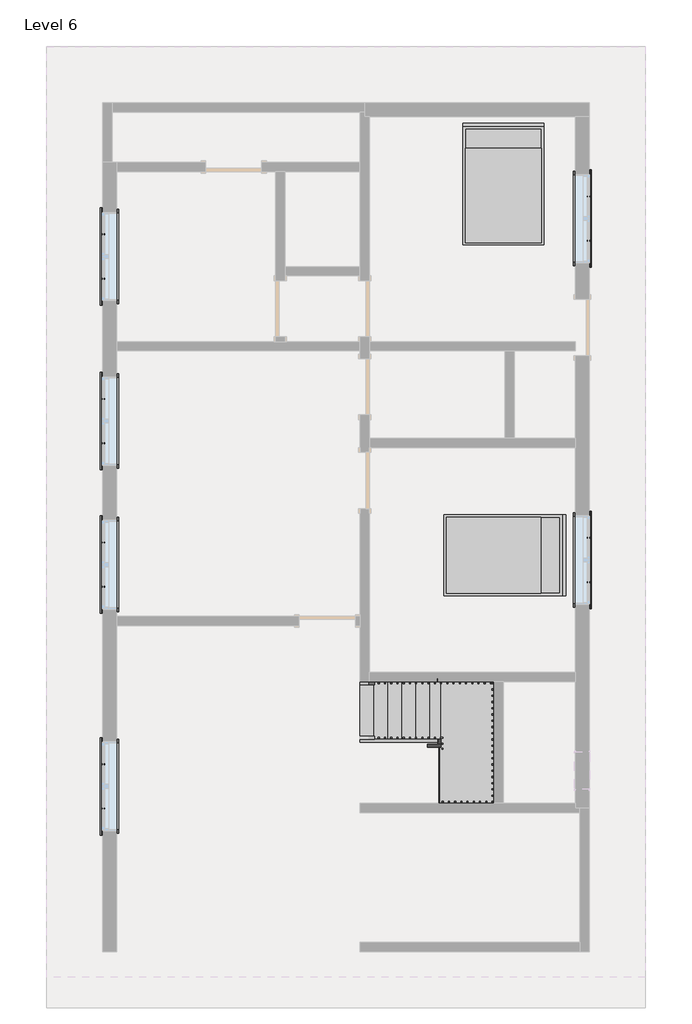
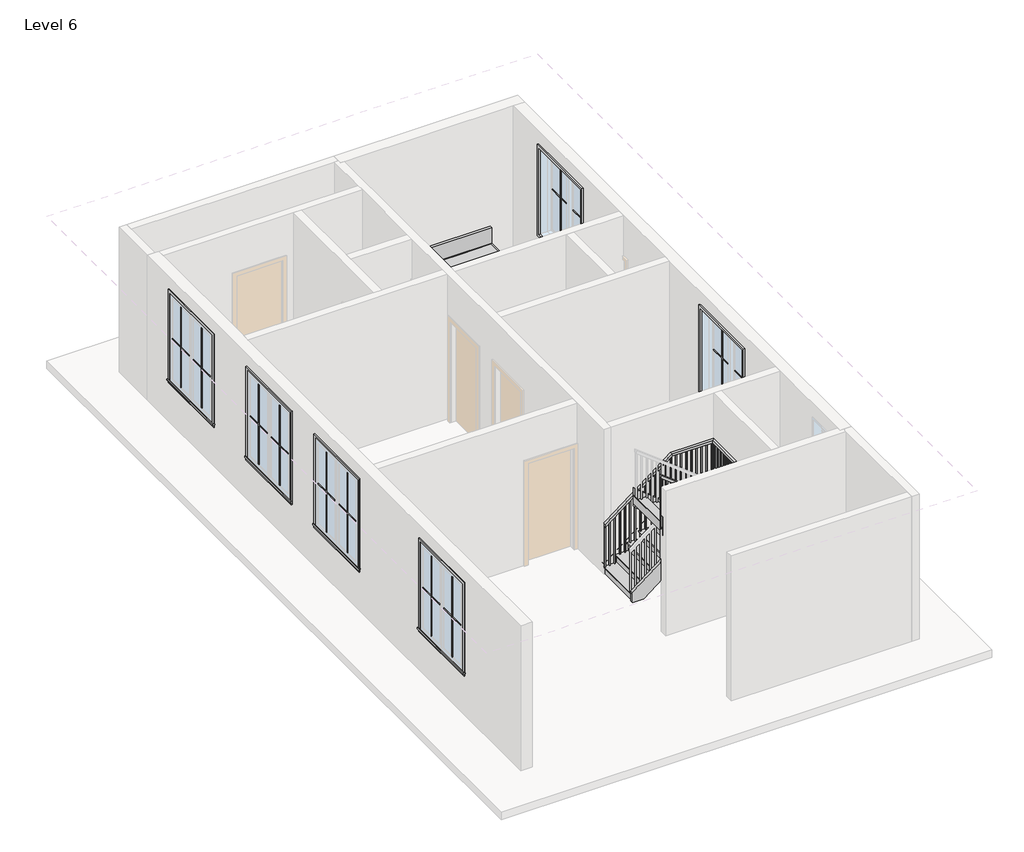
# One storey, part 2 of 2: 24 proxies, 6 members, 2 furniture elements, 1 railing, 1 stair flight.
"""IFC4 building model written with IfcOpenShell, lengths in millimetres."""

from ifc_helpers import new_model, si_unit, frame, origin, place, context, project, spatial, polyline, outline, extrude, faceted_brep, transform, mapped, element, save
from components import muntin_pattern_2x2_muntin_pattern_2x2_bff912c5, muntin_pattern_2x2_muntin_pattern_2x2_c2194282, trim_window_exterior_flat_with_sill_e04b3088, trim_window_interior_flat_picture_frame_2a7685fe, bed_17739_bed_17739_15c61121, stair_flight_b066332a

model = new_model("IFC4")

# Units and contexts
model_context = context("Model", 3, world=origin())
ifc_project = project(units=[si_unit("LENGTHUNIT", "METRE", prefix="MILLI")], contexts=[model_context])

# Site, building, storey
site = spatial("IfcSite", under=ifc_project)
building = spatial("IfcBuilding", under=site)
storey = spatial("IfcBuildingStorey", under=building, Name="Level 6", Elevation=12801.6)

# Proxies
placement = place(None, origin())
muntin_pattern_2x2_muntin_pattern_2x2_shape = muntin_pattern_2x2_muntin_pattern_2x2_bff912c5(model_context)
element("IfcBuildingElementProxy", 1, Name="Muntin Pattern_2x2 : Muntin Pattern_2x2", ObjectType="Muntin Pattern_2x2 : Muntin Pattern_2x2", at=placement, inside=storey, context=model_context, shape_type="MappedRepresentation", body=[
    mapped(muntin_pattern_2x2_muntin_pattern_2x2_shape, transform((-5204.1165352, 3633.8812696, 13785.85), x_axis=(0.0, 1.0, 0.0), y_axis=(-1.0, 0.0, 0.0), z_axis=(0.0, 0.0, 1.0))),
])
element("IfcBuildingElementProxy", 2, Name="Muntin Pattern_2x2 : Muntin Pattern_2x2", ObjectType="Muntin Pattern_2x2 : Muntin Pattern_2x2", at=placement, inside=storey, context=model_context, shape_type="MappedRepresentation", body=[
    mapped(muntin_pattern_2x2_muntin_pattern_2x2_shape, transform((2701.6334648, 4971.3355313, 13785.85), x_axis=(0.0, -1.0, 0.0), y_axis=(1.0, 0.0, 0.0), z_axis=(0.0, 0.0, 1.0))),
])
element("IfcBuildingElementProxy", 3, Name="Muntin Pattern_2x2 : Muntin Pattern_2x2", ObjectType="Muntin Pattern_2x2 : Muntin Pattern_2x2", at=placement, inside=storey, context=model_context, shape_type="MappedRepresentation", body=[
    mapped(muntin_pattern_2x2_muntin_pattern_2x2_shape, transform((2701.6334648, -584.9144687, 13785.85), x_axis=(0.0, -1.0, 0.0), y_axis=(1.0, 0.0, 0.0), z_axis=(0.0, 0.0, 1.0))),
])
element("IfcBuildingElementProxy", 4, Name="Muntin Pattern_2x2 : Muntin Pattern_2x2", ObjectType="Muntin Pattern_2x2 : Muntin Pattern_2x2", at=placement, inside=storey, context=model_context, shape_type="MappedRepresentation", body=[
    mapped(muntin_pattern_2x2_muntin_pattern_2x2_shape, transform((-5204.1165352, 954.9605313, 13785.85), x_axis=(0.0, 1.0, 0.0), y_axis=(-1.0, 0.0, 0.0), z_axis=(0.0, 0.0, 1.0))),
])
element("IfcBuildingElementProxy", 5, Name="Muntin Pattern_2x2 : Muntin Pattern_2x2", ObjectType="Muntin Pattern_2x2 : Muntin Pattern_2x2", at=placement, inside=storey, context=model_context, shape_type="MappedRepresentation", body=[
    mapped(muntin_pattern_2x2_muntin_pattern_2x2_shape, transform((-5204.1165352, -1381.8394687, 13785.85), x_axis=(0.0, 1.0, 0.0), y_axis=(-1.0, 0.0, 0.0), z_axis=(0.0, 0.0, 1.0))),
])
element("IfcBuildingElementProxy", 6, Name="Muntin Pattern_2x2 : Muntin Pattern_2x2", ObjectType="Muntin Pattern_2x2 : Muntin Pattern_2x2", at=placement, inside=storey, context=model_context, shape_type="MappedRepresentation", body=[
    mapped(muntin_pattern_2x2_muntin_pattern_2x2_shape, transform((-5204.1165352, -4988.6394687, 13785.85), x_axis=(0.0, 1.0, 0.0), y_axis=(-1.0, 0.0, 0.0), z_axis=(0.0, 0.0, 1.0))),
])
muntin_pattern_2x2_muntin_pattern_2x2_2_shape = muntin_pattern_2x2_muntin_pattern_2x2_c2194282(model_context)
element("IfcBuildingElementProxy", 7, Name="Muntin Pattern_2x2 : Muntin Pattern_2x2", ObjectType="Muntin Pattern_2x2 : Muntin Pattern_2x2", at=placement, inside=storey, context=model_context, shape_type="MappedRepresentation", body=[
    mapped(muntin_pattern_2x2_muntin_pattern_2x2_2_shape, transform((-5204.1165352, 4354.6062696, 13785.85), x_axis=(0.0, -1.0, 0.0), y_axis=(1.0, 0.0, 0.0), z_axis=(0.0, 0.0, 1.0))),
])
element("IfcBuildingElementProxy", 8, Name="Muntin Pattern_2x2 : Muntin Pattern_2x2", ObjectType="Muntin Pattern_2x2 : Muntin Pattern_2x2", at=placement, inside=storey, context=model_context, shape_type="MappedRepresentation", body=[
    mapped(muntin_pattern_2x2_muntin_pattern_2x2_2_shape, transform((2701.6334648, 4250.6105313, 13785.85), x_axis=(0.0, 1.0, 0.0), y_axis=(-1.0, 0.0, 0.0), z_axis=(0.0, 0.0, 1.0))),
])
element("IfcBuildingElementProxy", 9, Name="Muntin Pattern_2x2 : Muntin Pattern_2x2", ObjectType="Muntin Pattern_2x2 : Muntin Pattern_2x2", at=placement, inside=storey, context=model_context, shape_type="MappedRepresentation", body=[
    mapped(muntin_pattern_2x2_muntin_pattern_2x2_2_shape, transform((2701.6334648, -1305.6394687, 13785.85), x_axis=(0.0, 1.0, 0.0), y_axis=(-1.0, 0.0, 0.0), z_axis=(0.0, 0.0, 1.0))),
])
element("IfcBuildingElementProxy", 10, Name="Muntin Pattern_2x2 : Muntin Pattern_2x2", ObjectType="Muntin Pattern_2x2 : Muntin Pattern_2x2", at=placement, inside=storey, context=model_context, shape_type="MappedRepresentation", body=[
    mapped(muntin_pattern_2x2_muntin_pattern_2x2_2_shape, transform((-5204.1165352, 1675.6855313, 13785.85), x_axis=(0.0, -1.0, 0.0), y_axis=(1.0, 0.0, 0.0), z_axis=(0.0, 0.0, 1.0))),
])
element("IfcBuildingElementProxy", 11, Name="Muntin Pattern_2x2 : Muntin Pattern_2x2", ObjectType="Muntin Pattern_2x2 : Muntin Pattern_2x2", at=placement, inside=storey, context=model_context, shape_type="MappedRepresentation", body=[
    mapped(muntin_pattern_2x2_muntin_pattern_2x2_2_shape, transform((-5204.1165352, -661.1144687, 13785.85), x_axis=(0.0, -1.0, 0.0), y_axis=(1.0, 0.0, 0.0), z_axis=(0.0, 0.0, 1.0))),
])
element("IfcBuildingElementProxy", 12, Name="Muntin Pattern_2x2 : Muntin Pattern_2x2", ObjectType="Muntin Pattern_2x2 : Muntin Pattern_2x2", at=placement, inside=storey, context=model_context, shape_type="MappedRepresentation", body=[
    mapped(muntin_pattern_2x2_muntin_pattern_2x2_2_shape, transform((-5204.1165352, -4267.9144687, 13785.85), x_axis=(0.0, -1.0, 0.0), y_axis=(1.0, 0.0, 0.0), z_axis=(0.0, 0.0, 1.0))),
])
trim_window_exterior_flat_with_sill_shape = trim_window_exterior_flat_with_sill_e04b3088(model_context)
element("IfcBuildingElementProxy", 13, Name="Trim-Window-Exterior-Flat : with Sill", ObjectType="Trim-Window-Exterior-Flat : with Sill", at=placement, inside=storey, context=model_context, shape_type="MappedRepresentation", body=[
    mapped(trim_window_exterior_flat_with_sill_shape, transform((-5213.6415352, 3994.2437696, 15544.8), x_axis=(0.0, -1.0, 0.0), y_axis=(0.0, 0.0, 1.0), z_axis=(-1.0, 0.0, 0.0))),
])
element("IfcBuildingElementProxy", 14, Name="Trim-Window-Exterior-Flat : with Sill", ObjectType="Trim-Window-Exterior-Flat : with Sill", at=placement, inside=storey, context=model_context, shape_type="MappedRepresentation", body=[
    mapped(trim_window_exterior_flat_with_sill_shape, transform((2711.1584648, 4610.9730313, 15544.8), x_axis=(0.0, 1.0, 0.0), y_axis=(0.0, 0.0, 1.0), z_axis=(1.0, 0.0, 0.0))),
])
element("IfcBuildingElementProxy", 15, Name="Trim-Window-Exterior-Flat : with Sill", ObjectType="Trim-Window-Exterior-Flat : with Sill", at=placement, inside=storey, context=model_context, shape_type="MappedRepresentation", body=[
    mapped(trim_window_exterior_flat_with_sill_shape, transform((2711.1584648, -945.2769687, 15544.8), x_axis=(0.0, 1.0, 0.0), y_axis=(0.0, 0.0, 1.0), z_axis=(1.0, 0.0, 0.0))),
])
element("IfcBuildingElementProxy", 16, Name="Trim-Window-Exterior-Flat : with Sill", ObjectType="Trim-Window-Exterior-Flat : with Sill", at=placement, inside=storey, context=model_context, shape_type="MappedRepresentation", body=[
    mapped(trim_window_exterior_flat_with_sill_shape, transform((-5213.6415352, 1315.3230313, 15544.8), x_axis=(0.0, -1.0, 0.0), y_axis=(0.0, 0.0, 1.0), z_axis=(-1.0, 0.0, 0.0))),
])
element("IfcBuildingElementProxy", 17, Name="Trim-Window-Exterior-Flat : with Sill", ObjectType="Trim-Window-Exterior-Flat : with Sill", at=placement, inside=storey, context=model_context, shape_type="MappedRepresentation", body=[
    mapped(trim_window_exterior_flat_with_sill_shape, transform((-5213.6415352, -1021.4769687, 15544.8), x_axis=(0.0, -1.0, 0.0), y_axis=(0.0, 0.0, 1.0), z_axis=(-1.0, 0.0, 0.0))),
])
element("IfcBuildingElementProxy", 18, Name="Trim-Window-Exterior-Flat : with Sill", ObjectType="Trim-Window-Exterior-Flat : with Sill", at=placement, inside=storey, context=model_context, shape_type="MappedRepresentation", body=[
    mapped(trim_window_exterior_flat_with_sill_shape, transform((-5213.6415352, -4628.2769687, 15544.8), x_axis=(0.0, -1.0, 0.0), y_axis=(0.0, 0.0, 1.0), z_axis=(-1.0, 0.0, 0.0))),
])
trim_window_interior_flat_picture_frame_shape = trim_window_interior_flat_picture_frame_2a7685fe(model_context)
element("IfcBuildingElementProxy", 19, Name="Trim-Window-Interior-Flat : Picture Frame", ObjectType="Trim-Window-Interior-Flat : Picture Frame", at=placement, inside=storey, context=model_context, shape_type="MappedRepresentation", body=[
    mapped(trim_window_interior_flat_picture_frame_shape, transform((-4985.0415352, 3994.2437696, 15544.8), x_axis=(0.0, 1.0, 0.0), y_axis=(0.0, 0.0, 1.0), z_axis=(1.0, 0.0, 0.0))),
])
element("IfcBuildingElementProxy", 20, Name="Trim-Window-Interior-Flat : Picture Frame", ObjectType="Trim-Window-Interior-Flat : Picture Frame", at=placement, inside=storey, context=model_context, shape_type="MappedRepresentation", body=[
    mapped(trim_window_interior_flat_picture_frame_shape, transform((2482.5584648, 4610.9730313, 15544.8), x_axis=(0.0, -1.0, 0.0), y_axis=(0.0, 0.0, 1.0), z_axis=(-1.0, 0.0, 0.0))),
])
element("IfcBuildingElementProxy", 21, Name="Trim-Window-Interior-Flat : Picture Frame", ObjectType="Trim-Window-Interior-Flat : Picture Frame", at=placement, inside=storey, context=model_context, shape_type="MappedRepresentation", body=[
    mapped(trim_window_interior_flat_picture_frame_shape, transform((2482.5584648, -945.2769687, 15544.8), x_axis=(0.0, -1.0, 0.0), y_axis=(0.0, 0.0, 1.0), z_axis=(-1.0, 0.0, 0.0))),
])
element("IfcBuildingElementProxy", 22, Name="Trim-Window-Interior-Flat : Picture Frame", ObjectType="Trim-Window-Interior-Flat : Picture Frame", at=placement, inside=storey, context=model_context, shape_type="MappedRepresentation", body=[
    mapped(trim_window_interior_flat_picture_frame_shape, transform((-4985.0415352, 1315.3230313, 15544.8), x_axis=(0.0, 1.0, 0.0), y_axis=(0.0, 0.0, 1.0), z_axis=(1.0, 0.0, 0.0))),
])
element("IfcBuildingElementProxy", 23, Name="Trim-Window-Interior-Flat : Picture Frame", ObjectType="Trim-Window-Interior-Flat : Picture Frame", at=placement, inside=storey, context=model_context, shape_type="MappedRepresentation", body=[
    mapped(trim_window_interior_flat_picture_frame_shape, transform((-4985.0415352, -1021.4769687, 15544.8), x_axis=(0.0, 1.0, 0.0), y_axis=(0.0, 0.0, 1.0), z_axis=(1.0, 0.0, 0.0))),
])
element("IfcBuildingElementProxy", 24, Name="Trim-Window-Interior-Flat : Picture Frame", ObjectType="Trim-Window-Interior-Flat : Picture Frame", at=placement, inside=storey, context=model_context, shape_type="MappedRepresentation", body=[
    mapped(trim_window_interior_flat_picture_frame_shape, transform((-4985.0415352, -4628.2769687, 15544.8), x_axis=(0.0, 1.0, 0.0), y_axis=(0.0, 0.0, 1.0), z_axis=(1.0, 0.0, 0.0))),
])

# Furniture
bed_17739_bed_17739_shape = bed_17739_bed_17739_15c61121(model_context)
element("IfcFurniture", 25, ObjectType="Bed_17739 : Bed_17739", at=placement, inside=storey, context=model_context, shape_type="MappedRepresentation", body=[
    mapped(bed_17739_bed_17739_shape, transform((1314.1584648, 5149.1645078, 12801.6), x_axis=(1.0, 0.0, 0.0), y_axis=(0.0, 1.0, 0.0), z_axis=(0.0, 0.0, 1.0))),
])
element("IfcFurniture", 26, ObjectType="Bed_17739 : Bed_17739", at=placement, inside=storey, context=model_context, shape_type="MappedRepresentation", body=[
    mapped(bed_17739_bed_17739_shape, transform((1314.1584648, -869.0769687, 12801.6), x_axis=(0.0, -1.0, 0.0), y_axis=(1.0, 0.0, 0.0), z_axis=(0.0, 0.0, 1.0))),
])

# Members
element("IfcMember", 27, ObjectType="Stringer - 2\" Width", at=placement, inside=storey, context=model_context, shape_type="SweptSolid", body=[
    extrude(outline(polyline([(13023.3399812, -1022.6415352), (12801.6, -1022.6415352), (12801.6, -811.2687863), (14063.1333333, 810.8400359), (14063.1333333, 314.3488758), (13023.3399812, -1022.6415352)])), frame((0.0, -2926.4769687, 0.0), z_axis=(0.0, 1.0, 0.0), x_axis=(0.0, 0.0, 1.0)), (0.0, 0.0, 1.0), 50.8),
])
element("IfcMember", 28, ObjectType="Stringer - 2\" Width", at=placement, inside=storey, context=model_context, shape_type="SweptSolid", body=[
    extrude(outline(polyline([(1161.7584648, -2875.6769687), (1212.5584648, -2875.6769687), (1212.5584648, -4907.6769687), (1161.7584648, -4907.6769687), (1161.7584648, -2875.6769687)])), frame((0.0, 0.0, 13758.3333333), z_axis=(0.0, 0.0, 1.0), x_axis=(1.0, 0.0, 0.0)), (0.0, 0.0, 1.0), 304.8),
])
element("IfcMember", 29, ObjectType="Stringer - 2\" Width", at=placement, inside=storey, context=model_context, shape_type="SweptSolid", body=[
    extrude(outline(polyline([(13758.3333333, 884.5469698), (15241.5765283, -1022.6415352), (14855.4494451, -1022.6415352), (13758.3333333, 388.0558097), (13758.3333333, 884.5469698)])), frame((0.0, -4958.4769687, 0.0), z_axis=(0.0, 1.0, 0.0), x_axis=(0.0, 0.0, 1.0)), (0.0, 0.0, 1.0), 50.8),
])
element("IfcMember", 30, ObjectType="Stringer - 2\" Width", at=placement, inside=storey, context=model_context, shape_type="SweptSolid", body=[
    extrude(outline(polyline([(13023.3399812, -1022.6415352), (12801.6, -1022.6415352), (12801.6, -811.2687863), (13622.1567404, 243.8221038), (14008.2838236, 243.8221038), (13023.3399812, -1022.6415352)])), frame((0.0, -3912.0539367, 0.0), z_axis=(0.0, 1.0, 0.0), x_axis=(0.0, 0.0, 1.0)), (0.0, 0.0, 1.0), 50.8),
])
element("IfcMember", 31, ObjectType="Stringer - 2\" Width", at=placement, inside=storey, context=model_context, shape_type="SweptSolid", body=[
    extrude(outline(polyline([(243.8221038, -3861.2539367), (294.6221038, -3861.2539367), (294.6221038, -3942.4769687), (243.8221038, -3942.4769687), (243.8221038, -3861.2539367)])), frame((0.0, 0.0, 13758.3333333), z_axis=(0.0, 0.0, 1.0), x_axis=(1.0, 0.0, 0.0)), (0.0, 0.0, 1.0), 304.8),
])
element("IfcMember", 32, ObjectType="Stringer - 2\" Width", at=placement, inside=storey, context=model_context, shape_type="SweptSolid", body=[
    extrude(outline(polyline([(13830.9978382, 294.6221038), (14217.1249214, 294.6221038), (15241.5765283, -1022.6415352), (14855.4494451, -1022.6415352), (13830.9978382, 294.6221038)])), frame((0.0, -3993.2769687, 0.0), z_axis=(0.0, 1.0, 0.0), x_axis=(0.0, 0.0, 1.0)), (0.0, 0.0, 1.0), 50.8),
])

# Railing
element("IfcRailing", 33, ObjectType="Handrail - Rectangular", at=placement, inside=storey, context=model_context, shape_type="SolidModel", body=[
    faceted_brep([(-1022.6415352, -2926.4769687, 13885.3333333), (-1022.6415352, -2926.4769687, 13821.1783974), (-1022.6415352, -2977.2769687, 13821.1783974), (-1022.6415352, -2977.2769687, 13885.3333333), (294.6221038, -2926.4769687, 14901.3333333), (311.9370364, -2926.4769687, 14850.5333333), (311.9370364, -2977.2769687, 14850.5333333), (294.6221038, -2977.2769687, 14901.3333333), (1161.7584648, -2926.4769687, 14901.3333333), (1161.7584648, -2926.4769687, 14850.5333333), (1110.9584648, -2977.2769687, 14850.5333333), (1110.9584648, -2977.2769687, 14901.3333333), (1161.7584648, -4907.6769687, 14901.3333333), (1161.7584648, -4907.6769687, 14850.5333333), (1110.9584648, -4856.8769687, 14850.5333333), (1110.9584648, -4856.8769687, 14901.3333333), (514.1660437, -4907.6769687, 14901.3333333), (496.8511111, -4907.6769687, 14850.5333333), (496.8511111, -4856.8769687, 14850.5333333), (514.1660437, -4856.8769687, 14901.3333333), (-1022.6415352, -4907.6769687, 16086.6666667), (-1022.6415352, -4856.8769687, 16086.6666667), (-1022.6415352, -4856.8769687, 16022.5117307), (-1022.6415352, -4907.6769687, 16022.5117307)], [[[0, 1, 2, 3]], [[1, 0, 4, 5]], [[2, 1, 5, 6]], [[3, 2, 6, 7]], [[0, 3, 7, 4]], [[5, 4, 8, 9]], [[6, 5, 9, 10]], [[7, 6, 10, 11]], [[4, 7, 11, 8]], [[9, 8, 12, 13]], [[10, 9, 13, 14]], [[11, 10, 14, 15]], [[8, 11, 15, 12]], [[13, 12, 16, 17]], [[14, 13, 17, 18]], [[15, 14, 18, 19]], [[12, 15, 19, 16]], [[20, 21, 22, 23]], [[17, 16, 20, 23]], [[18, 17, 23, 22]], [[19, 18, 22, 21]], [[16, 19, 21, 20]]]),
    extrude(outline(polyline([(16010.2674089, -1006.7665352), (15002.9333333, -1006.7665352), (15002.9333333, -987.7165352), (15995.5742226, -987.7165352), (16010.2674089, -1006.7665352)])), frame((0.0, -4891.8019687, 0.0), z_axis=(0.0, 1.0, 0.0), x_axis=(0.0, 0.0, 1.0)), (0.0, 0.0, 1.0), 19.05),
    extrude(outline(polyline([(15931.9037488, -905.1665352), (15002.9333333, -905.1665352), (15002.9333333, -886.1165352), (15917.2105626, -886.1165352), (15931.9037488, -905.1665352)])), frame((0.0, -4891.8019687, 0.0), z_axis=(0.0, 1.0, 0.0), x_axis=(0.0, 0.0, 1.0)), (0.0, 0.0, 1.0), 19.05),
    extrude(outline(polyline([(15853.5400888, -803.5665352), (15002.9333333, -803.5665352), (15002.9333333, -784.5165352), (15838.8469025, -784.5165352), (15853.5400888, -803.5665352)])), frame((0.0, -4891.8019687, 0.0), z_axis=(0.0, 1.0, 0.0), x_axis=(0.0, 0.0, 1.0)), (0.0, 0.0, 1.0), 19.05),
    extrude(outline(polyline([(15775.1764287, -701.9665352), (14833.6, -701.9665352), (14833.6, -682.9165352), (15760.4832425, -682.9165352), (15775.1764287, -701.9665352)])), frame((0.0, -4891.8019687, 0.0), z_axis=(0.0, 1.0, 0.0), x_axis=(0.0, 0.0, 1.0)), (0.0, 0.0, 1.0), 19.05),
    extrude(outline(polyline([(15696.8127687, -600.3665352), (14833.6, -600.3665352), (14833.6, -581.3165352), (15682.1195824, -581.3165352), (15696.8127687, -600.3665352)])), frame((0.0, -4891.8019687, 0.0), z_axis=(0.0, 1.0, 0.0), x_axis=(0.0, 0.0, 1.0)), (0.0, 0.0, 1.0), 19.05),
    extrude(outline(polyline([(15618.4491086, -498.7665352), (14664.2666667, -498.7665352), (14664.2666667, -479.7165352), (15603.7559224, -479.7165352), (15618.4491086, -498.7665352)])), frame((0.0, -4891.8019687, 0.0), z_axis=(0.0, 1.0, 0.0), x_axis=(0.0, 0.0, 1.0)), (0.0, 0.0, 1.0), 19.05),
    extrude(outline(polyline([(15540.0854486, -397.1665352), (14664.2666667, -397.1665352), (14664.2666667, -378.1165352), (15525.3922623, -378.1165352), (15540.0854486, -397.1665352)])), frame((0.0, -4891.8019687, 0.0), z_axis=(0.0, 1.0, 0.0), x_axis=(0.0, 0.0, 1.0)), (0.0, 0.0, 1.0), 19.05),
    extrude(outline(polyline([(15461.7217885, -295.5665352), (14494.9333333, -295.5665352), (14494.9333333, -276.5165352), (15447.0286023, -276.5165352), (15461.7217885, -295.5665352)])), frame((0.0, -4891.8019687, 0.0), z_axis=(0.0, 1.0, 0.0), x_axis=(0.0, 0.0, 1.0)), (0.0, 0.0, 1.0), 19.05),
    extrude(outline(polyline([(15383.3581285, -193.9665352), (14494.9333333, -193.9665352), (14494.9333333, -174.9165352), (15368.6649422, -174.9165352), (15383.3581285, -193.9665352)])), frame((0.0, -4891.8019687, 0.0), z_axis=(0.0, 1.0, 0.0), x_axis=(0.0, 0.0, 1.0)), (0.0, 0.0, 1.0), 19.05),
    extrude(outline(polyline([(15304.9944684, -92.3665352), (14325.6, -92.3665352), (14325.6, -73.3165352), (15290.3012822, -73.3165352), (15304.9944684, -92.3665352)])), frame((0.0, -4891.8019687, 0.0), z_axis=(0.0, 1.0, 0.0), x_axis=(0.0, 0.0, 1.0)), (0.0, 0.0, 1.0), 19.05),
    extrude(outline(polyline([(15226.6308084, 9.2334648), (14325.6, 9.2334648), (14325.6, 28.2834648), (15211.9376221, 28.2834648), (15226.6308084, 9.2334648)])), frame((0.0, -4891.8019687, 0.0), z_axis=(0.0, 1.0, 0.0), x_axis=(0.0, 0.0, 1.0)), (0.0, 0.0, 1.0), 19.05),
    extrude(outline(polyline([(15148.2671484, 110.8334648), (14325.6, 110.8334648), (14325.6, 129.8834648), (15133.5739621, 129.8834648), (15148.2671484, 110.8334648)])), frame((0.0, -4891.8019687, 0.0), z_axis=(0.0, 1.0, 0.0), x_axis=(0.0, 0.0, 1.0)), (0.0, 0.0, 1.0), 19.05),
    extrude(outline(polyline([(15069.9034883, 212.4334648), (14156.2666667, 212.4334648), (14156.2666667, 231.4834648), (15055.2103021, 231.4834648), (15069.9034883, 212.4334648)])), frame((0.0, -4891.8019687, 0.0), z_axis=(0.0, 1.0, 0.0), x_axis=(0.0, 0.0, 1.0)), (0.0, 0.0, 1.0), 19.05),
    extrude(outline(polyline([(14991.5398283, 314.0334648), (13986.9333333, 314.0334648), (13986.9333333, 333.0834648), (14976.846642, 333.0834648), (14991.5398283, 314.0334648)])), frame((0.0, -4891.8019687, 0.0), z_axis=(0.0, 1.0, 0.0), x_axis=(0.0, 0.0, 1.0)), (0.0, 0.0, 1.0), 19.05),
    extrude(outline(polyline([(14913.1761682, 415.6334648), (13986.9333333, 415.6334648), (13986.9333333, 434.6834648), (14898.482982, 434.6834648), (14913.1761682, 415.6334648)])), frame((0.0, -4891.8019687, 0.0), z_axis=(0.0, 1.0, 0.0), x_axis=(0.0, 0.0, 1.0)), (0.0, 0.0, 1.0), 19.05),
    extrude(outline(polyline([(536.2834648, -4891.8019687), (517.2334648, -4891.8019687), (517.2334648, -4872.7519687), (536.2834648, -4872.7519687), (536.2834648, -4891.8019687)])), frame((0.0, 0.0, 13986.9333333), z_axis=(0.0, 0.0, 1.0), x_axis=(1.0, 0.0, 0.0)), (0.0, 0.0, 1.0), 863.6),
    extrude(outline(polyline([(637.8834648, -4891.8019687), (618.8334648, -4891.8019687), (618.8334648, -4872.7519687), (637.8834648, -4872.7519687), (637.8834648, -4891.8019687)])), frame((0.0, 0.0, 13986.9333333), z_axis=(0.0, 0.0, 1.0), x_axis=(1.0, 0.0, 0.0)), (0.0, 0.0, 1.0), 863.6),
    extrude(outline(polyline([(739.4834648, -4891.8019687), (720.4334648, -4891.8019687), (720.4334648, -4872.7519687), (739.4834648, -4872.7519687), (739.4834648, -4891.8019687)])), frame((0.0, 0.0, 13986.9333333), z_axis=(0.0, 0.0, 1.0), x_axis=(1.0, 0.0, 0.0)), (0.0, 0.0, 1.0), 863.6),
    extrude(outline(polyline([(841.0834648, -4891.8019687), (822.0334648, -4891.8019687), (822.0334648, -4872.7519687), (841.0834648, -4872.7519687), (841.0834648, -4891.8019687)])), frame((0.0, 0.0, 13986.9333333), z_axis=(0.0, 0.0, 1.0), x_axis=(1.0, 0.0, 0.0)), (0.0, 0.0, 1.0), 863.6),
    extrude(outline(polyline([(942.6834648, -4891.8019687), (923.6334648, -4891.8019687), (923.6334648, -4872.7519687), (942.6834648, -4872.7519687), (942.6834648, -4891.8019687)])), frame((0.0, 0.0, 13986.9333333), z_axis=(0.0, 0.0, 1.0), x_axis=(1.0, 0.0, 0.0)), (0.0, 0.0, 1.0), 863.6),
    extrude(outline(polyline([(1044.2834648, -4891.8019687), (1025.2334648, -4891.8019687), (1025.2334648, -4872.7519687), (1044.2834648, -4872.7519687), (1044.2834648, -4891.8019687)])), frame((0.0, 0.0, 13986.9333333), z_axis=(0.0, 0.0, 1.0), x_axis=(1.0, 0.0, 0.0)), (0.0, 0.0, 1.0), 863.6),
    extrude(outline(polyline([(1145.8834648, -4771.1519687), (1145.8834648, -4790.2019687), (1126.8334648, -4790.2019687), (1126.8334648, -4771.1519687), (1145.8834648, -4771.1519687)])), frame((0.0, 0.0, 13986.9333333), z_axis=(0.0, 0.0, 1.0), x_axis=(1.0, 0.0, 0.0)), (0.0, 0.0, 1.0), 863.6),
    extrude(outline(polyline([(1145.8834648, -4669.5519687), (1145.8834648, -4688.6019687), (1126.8334648, -4688.6019687), (1126.8334648, -4669.5519687), (1145.8834648, -4669.5519687)])), frame((0.0, 0.0, 13986.9333333), z_axis=(0.0, 0.0, 1.0), x_axis=(1.0, 0.0, 0.0)), (0.0, 0.0, 1.0), 863.6),
    extrude(outline(polyline([(1145.8834648, -4567.9519687), (1145.8834648, -4587.0019687), (1126.8334648, -4587.0019687), (1126.8334648, -4567.9519687), (1145.8834648, -4567.9519687)])), frame((0.0, 0.0, 13986.9333333), z_axis=(0.0, 0.0, 1.0), x_axis=(1.0, 0.0, 0.0)), (0.0, 0.0, 1.0), 863.6),
    extrude(outline(polyline([(1145.8834648, -4466.3519687), (1145.8834648, -4485.4019687), (1126.8334648, -4485.4019687), (1126.8334648, -4466.3519687), (1145.8834648, -4466.3519687)])), frame((0.0, 0.0, 13986.9333333), z_axis=(0.0, 0.0, 1.0), x_axis=(1.0, 0.0, 0.0)), (0.0, 0.0, 1.0), 863.6),
    extrude(outline(polyline([(1145.8834648, -4364.7519687), (1145.8834648, -4383.8019687), (1126.8334648, -4383.8019687), (1126.8334648, -4364.7519687), (1145.8834648, -4364.7519687)])), frame((0.0, 0.0, 13986.9333333), z_axis=(0.0, 0.0, 1.0), x_axis=(1.0, 0.0, 0.0)), (0.0, 0.0, 1.0), 863.6),
    extrude(outline(polyline([(1145.8834648, -4263.1519687), (1145.8834648, -4282.2019687), (1126.8334648, -4282.2019687), (1126.8334648, -4263.1519687), (1145.8834648, -4263.1519687)])), frame((0.0, 0.0, 13986.9333333), z_axis=(0.0, 0.0, 1.0), x_axis=(1.0, 0.0, 0.0)), (0.0, 0.0, 1.0), 863.6),
    extrude(outline(polyline([(1145.8834648, -4161.5519687), (1145.8834648, -4180.6019687), (1126.8334648, -4180.6019687), (1126.8334648, -4161.5519687), (1145.8834648, -4161.5519687)])), frame((0.0, 0.0, 13986.9333333), z_axis=(0.0, 0.0, 1.0), x_axis=(1.0, 0.0, 0.0)), (0.0, 0.0, 1.0), 863.6),
    extrude(outline(polyline([(1145.8834648, -4059.9519687), (1145.8834648, -4079.0019687), (1126.8334648, -4079.0019687), (1126.8334648, -4059.9519687), (1145.8834648, -4059.9519687)])), frame((0.0, 0.0, 13986.9333333), z_axis=(0.0, 0.0, 1.0), x_axis=(1.0, 0.0, 0.0)), (0.0, 0.0, 1.0), 863.6),
    extrude(outline(polyline([(1145.8834648, -3958.3519687), (1145.8834648, -3977.4019687), (1126.8334648, -3977.4019687), (1126.8334648, -3958.3519687), (1145.8834648, -3958.3519687)])), frame((0.0, 0.0, 13986.9333333), z_axis=(0.0, 0.0, 1.0), x_axis=(1.0, 0.0, 0.0)), (0.0, 0.0, 1.0), 863.6),
    extrude(outline(polyline([(1145.8834648, -3856.7519687), (1145.8834648, -3875.8019687), (1126.8334648, -3875.8019687), (1126.8334648, -3856.7519687), (1145.8834648, -3856.7519687)])), frame((0.0, 0.0, 13986.9333333), z_axis=(0.0, 0.0, 1.0), x_axis=(1.0, 0.0, 0.0)), (0.0, 0.0, 1.0), 863.6),
    extrude(outline(polyline([(1145.8834648, -3755.1519687), (1145.8834648, -3774.2019687), (1126.8334648, -3774.2019687), (1126.8334648, -3755.1519687), (1145.8834648, -3755.1519687)])), frame((0.0, 0.0, 13986.9333333), z_axis=(0.0, 0.0, 1.0), x_axis=(1.0, 0.0, 0.0)), (0.0, 0.0, 1.0), 863.6),
    extrude(outline(polyline([(1145.8834648, -3653.5519687), (1145.8834648, -3672.6019687), (1126.8334648, -3672.6019687), (1126.8334648, -3653.5519687), (1145.8834648, -3653.5519687)])), frame((0.0, 0.0, 13986.9333333), z_axis=(0.0, 0.0, 1.0), x_axis=(1.0, 0.0, 0.0)), (0.0, 0.0, 1.0), 863.6),
    extrude(outline(polyline([(1145.8834648, -3551.9519687), (1145.8834648, -3571.0019687), (1126.8334648, -3571.0019687), (1126.8334648, -3551.9519687), (1145.8834648, -3551.9519687)])), frame((0.0, 0.0, 13986.9333333), z_axis=(0.0, 0.0, 1.0), x_axis=(1.0, 0.0, 0.0)), (0.0, 0.0, 1.0), 863.6),
    extrude(outline(polyline([(1145.8834648, -3450.3519687), (1145.8834648, -3469.4019687), (1126.8334648, -3469.4019687), (1126.8334648, -3450.3519687), (1145.8834648, -3450.3519687)])), frame((0.0, 0.0, 13986.9333333), z_axis=(0.0, 0.0, 1.0), x_axis=(1.0, 0.0, 0.0)), (0.0, 0.0, 1.0), 863.6),
    extrude(outline(polyline([(1145.8834648, -3348.7519687), (1145.8834648, -3367.8019687), (1126.8334648, -3367.8019687), (1126.8334648, -3348.7519687), (1145.8834648, -3348.7519687)])), frame((0.0, 0.0, 13986.9333333), z_axis=(0.0, 0.0, 1.0), x_axis=(1.0, 0.0, 0.0)), (0.0, 0.0, 1.0), 863.6),
    extrude(outline(polyline([(1145.8834648, -3247.1519687), (1145.8834648, -3266.2019687), (1126.8334648, -3266.2019687), (1126.8334648, -3247.1519687), (1145.8834648, -3247.1519687)])), frame((0.0, 0.0, 13986.9333333), z_axis=(0.0, 0.0, 1.0), x_axis=(1.0, 0.0, 0.0)), (0.0, 0.0, 1.0), 863.6),
    extrude(outline(polyline([(1145.8834648, -3145.5519687), (1145.8834648, -3164.6019687), (1126.8334648, -3164.6019687), (1126.8334648, -3145.5519687), (1145.8834648, -3145.5519687)])), frame((0.0, 0.0, 13986.9333333), z_axis=(0.0, 0.0, 1.0), x_axis=(1.0, 0.0, 0.0)), (0.0, 0.0, 1.0), 863.6),
    extrude(outline(polyline([(1145.8834648, -3043.9519687), (1145.8834648, -3063.0019687), (1126.8334648, -3063.0019687), (1126.8334648, -3043.9519687), (1145.8834648, -3043.9519687)])), frame((0.0, 0.0, 13986.9333333), z_axis=(0.0, 0.0, 1.0), x_axis=(1.0, 0.0, 0.0)), (0.0, 0.0, 1.0), 863.6),
    extrude(outline(polyline([(1101.4334648, -2942.3519687), (1120.4834648, -2942.3519687), (1120.4834648, -2961.4019687), (1101.4334648, -2961.4019687), (1101.4334648, -2942.3519687)])), frame((0.0, 0.0, 13986.9333333), z_axis=(0.0, 0.0, 1.0), x_axis=(1.0, 0.0, 0.0)), (0.0, 0.0, 1.0), 863.6),
    extrude(outline(polyline([(999.8334648, -2942.3519687), (1018.8834648, -2942.3519687), (1018.8834648, -2961.4019687), (999.8334648, -2961.4019687), (999.8334648, -2942.3519687)])), frame((0.0, 0.0, 13986.9333333), z_axis=(0.0, 0.0, 1.0), x_axis=(1.0, 0.0, 0.0)), (0.0, 0.0, 1.0), 863.6),
    extrude(outline(polyline([(898.2334648, -2942.3519687), (917.2834648, -2942.3519687), (917.2834648, -2961.4019687), (898.2334648, -2961.4019687), (898.2334648, -2942.3519687)])), frame((0.0, 0.0, 13986.9333333), z_axis=(0.0, 0.0, 1.0), x_axis=(1.0, 0.0, 0.0)), (0.0, 0.0, 1.0), 863.6),
    extrude(outline(polyline([(796.6334648, -2942.3519687), (815.6834648, -2942.3519687), (815.6834648, -2961.4019687), (796.6334648, -2961.4019687), (796.6334648, -2942.3519687)])), frame((0.0, 0.0, 13986.9333333), z_axis=(0.0, 0.0, 1.0), x_axis=(1.0, 0.0, 0.0)), (0.0, 0.0, 1.0), 863.6),
    extrude(outline(polyline([(695.0334648, -2942.3519687), (714.0834648, -2942.3519687), (714.0834648, -2961.4019687), (695.0334648, -2961.4019687), (695.0334648, -2942.3519687)])), frame((0.0, 0.0, 13986.9333333), z_axis=(0.0, 0.0, 1.0), x_axis=(1.0, 0.0, 0.0)), (0.0, 0.0, 1.0), 863.6),
    extrude(outline(polyline([(593.4334648, -2942.3519687), (612.4834648, -2942.3519687), (612.4834648, -2961.4019687), (593.4334648, -2961.4019687), (593.4334648, -2942.3519687)])), frame((0.0, 0.0, 13986.9333333), z_axis=(0.0, 0.0, 1.0), x_axis=(1.0, 0.0, 0.0)), (0.0, 0.0, 1.0), 863.6),
    extrude(outline(polyline([(491.8334648, -2942.3519687), (510.8834648, -2942.3519687), (510.8834648, -2961.4019687), (491.8334648, -2961.4019687), (491.8334648, -2942.3519687)])), frame((0.0, 0.0, 13986.9333333), z_axis=(0.0, 0.0, 1.0), x_axis=(1.0, 0.0, 0.0)), (0.0, 0.0, 1.0), 863.6),
    extrude(outline(polyline([(390.2334648, -2942.3519687), (409.2834648, -2942.3519687), (409.2834648, -2961.4019687), (390.2334648, -2961.4019687), (390.2334648, -2942.3519687)])), frame((0.0, 0.0, 13986.9333333), z_axis=(0.0, 0.0, 1.0), x_axis=(1.0, 0.0, 0.0)), (0.0, 0.0, 1.0), 863.6),
    extrude(outline(polyline([(288.6334648, -2942.3519687), (307.6834648, -2942.3519687), (307.6834648, -2961.4019687), (288.6334648, -2961.4019687), (288.6334648, -2942.3519687)])), frame((0.0, 0.0, 13986.9333333), z_axis=(0.0, 0.0, 1.0), x_axis=(1.0, 0.0, 0.0)), (0.0, 0.0, 1.0), 863.6),
    extrude(outline(polyline([(14754.1957248, 187.0334648), (13817.6, 187.0334648), (13817.6, 206.0834648), (14768.8889111, 206.0834648), (14754.1957248, 187.0334648)])), frame((0.0, -2961.4019687, 0.0), z_axis=(0.0, 1.0, 0.0), x_axis=(0.0, 0.0, 1.0)), (0.0, 0.0, 1.0), 19.05),
    extrude(outline(polyline([(14675.8320648, 85.4334648), (13648.2666667, 85.4334648), (13648.2666667, 104.4834648), (14690.525251, 104.4834648), (14675.8320648, 85.4334648)])), frame((0.0, -2961.4019687, 0.0), z_axis=(0.0, 1.0, 0.0), x_axis=(0.0, 0.0, 1.0)), (0.0, 0.0, 1.0), 19.05),
    extrude(outline(polyline([(14597.4684047, -16.1665352), (13648.2666667, -16.1665352), (13648.2666667, 2.8834648), (14612.161591, 2.8834648), (14597.4684047, -16.1665352)])), frame((0.0, -2961.4019687, 0.0), z_axis=(0.0, 1.0, 0.0), x_axis=(0.0, 0.0, 1.0)), (0.0, 0.0, 1.0), 19.05),
    extrude(outline(polyline([(14519.1047447, -117.7665352), (13648.2666667, -117.7665352), (13648.2666667, -98.7165352), (14533.7979309, -98.7165352), (14519.1047447, -117.7665352)])), frame((0.0, -2961.4019687, 0.0), z_axis=(0.0, 1.0, 0.0), x_axis=(0.0, 0.0, 1.0)), (0.0, 0.0, 1.0), 19.05),
    extrude(outline(polyline([(14440.7410846, -219.3665352), (13478.9333333, -219.3665352), (13478.9333333, -200.3165352), (14455.4342709, -200.3165352), (14440.7410846, -219.3665352)])), frame((0.0, -2961.4019687, 0.0), z_axis=(0.0, 1.0, 0.0), x_axis=(0.0, 0.0, 1.0)), (0.0, 0.0, 1.0), 19.05),
    extrude(outline(polyline([(14362.3774246, -320.9665352), (13478.9333333, -320.9665352), (13478.9333333, -301.9165352), (14377.0706109, -301.9165352), (14362.3774246, -320.9665352)])), frame((0.0, -2961.4019687, 0.0), z_axis=(0.0, 1.0, 0.0), x_axis=(0.0, 0.0, 1.0)), (0.0, 0.0, 1.0), 19.05),
    extrude(outline(polyline([(14284.0137645, -422.5665352), (13309.6, -422.5665352), (13309.6, -403.5165352), (14298.7069508, -403.5165352), (14284.0137645, -422.5665352)])), frame((0.0, -2961.4019687, 0.0), z_axis=(0.0, 1.0, 0.0), x_axis=(0.0, 0.0, 1.0)), (0.0, 0.0, 1.0), 19.05),
    extrude(outline(polyline([(14205.6501045, -524.1665352), (13309.6, -524.1665352), (13309.6, -505.1165352), (14220.3432908, -505.1165352), (14205.6501045, -524.1665352)])), frame((0.0, -2961.4019687, 0.0), z_axis=(0.0, 1.0, 0.0), x_axis=(0.0, 0.0, 1.0)), (0.0, 0.0, 1.0), 19.05),
    extrude(outline(polyline([(14127.2864445, -625.7665352), (13140.2666667, -625.7665352), (13140.2666667, -606.7165352), (14141.9796307, -606.7165352), (14127.2864445, -625.7665352)])), frame((0.0, -2961.4019687, 0.0), z_axis=(0.0, 1.0, 0.0), x_axis=(0.0, 0.0, 1.0)), (0.0, 0.0, 1.0), 19.05),
    extrude(outline(polyline([(14048.9227844, -727.3665352), (13140.2666667, -727.3665352), (13140.2666667, -708.3165352), (14063.6159707, -708.3165352), (14048.9227844, -727.3665352)])), frame((0.0, -2961.4019687, 0.0), z_axis=(0.0, 1.0, 0.0), x_axis=(0.0, 0.0, 1.0)), (0.0, 0.0, 1.0), 19.05),
    extrude(outline(polyline([(13970.5591244, -828.9665352), (12970.9333333, -828.9665352), (12970.9333333, -809.9165352), (13985.2523106, -809.9165352), (13970.5591244, -828.9665352)])), frame((0.0, -2961.4019687, 0.0), z_axis=(0.0, 1.0, 0.0), x_axis=(0.0, 0.0, 1.0)), (0.0, 0.0, 1.0), 19.05),
    extrude(outline(polyline([(13892.1954643, -930.5665352), (12970.9333333, -930.5665352), (12970.9333333, -911.5165352), (13906.8886506, -911.5165352), (13892.1954643, -930.5665352)])), frame((0.0, -2961.4019687, 0.0), z_axis=(0.0, 1.0, 0.0), x_axis=(0.0, 0.0, 1.0)), (0.0, 0.0, 1.0), 19.05),
    extrude(outline(polyline([(1145.8834648, -4872.7519687), (1145.8834648, -4891.8019687), (1126.8334648, -4891.8019687), (1126.8334648, -4872.7519687), (1145.8834648, -4872.7519687)])), frame((0.0, 0.0, 13986.9333333), z_axis=(0.0, 0.0, 1.0), x_axis=(1.0, 0.0, 0.0)), (0.0, 0.0, 1.0), 863.6),
    extrude(outline(polyline([(1126.8334648, -2942.3519687), (1145.8834648, -2942.3519687), (1145.8834648, -2961.4019687), (1126.8334648, -2961.4019687), (1126.8334648, -2942.3519687)])), frame((0.0, 0.0, 13986.9333333), z_axis=(0.0, 0.0, 1.0), x_axis=(1.0, 0.0, 0.0)), (0.0, 0.0, 1.0), 863.6),
    extrude(outline(polyline([(16022.5117307, -1022.6415352), (15002.9333333, -1022.6415352), (15002.9333333, -1003.5915352), (16007.8185445, -1003.5915352), (16022.5117307, -1022.6415352)])), frame((0.0, -4891.8019687, 0.0), z_axis=(0.0, 1.0, 0.0), x_axis=(0.0, 0.0, 1.0)), (0.0, 0.0, 1.0), 19.05),
    extrude(outline(polyline([(13821.1783974, -1022.6415352), (12970.9333333, -1022.6415352), (12970.9333333, -1003.5915352), (13835.8715837, -1003.5915352), (13821.1783974, -1022.6415352)])), frame((0.0, -2961.4019687, 0.0), z_axis=(0.0, 1.0, 0.0), x_axis=(0.0, 0.0, 1.0)), (0.0, 0.0, 1.0), 19.05),
])

# Stair flight
stair_flight_shape = stair_flight_b066332a(model_context)
element("IfcStairFlight", 34, ObjectType="2\" Tread 1\" Nosing 1/4\" Riser", at=placement, inside=storey, context=model_context, shape_type="MappedRepresentation", body=[
    mapped(stair_flight_shape, transform((0.0, 0.0, 0.0), x_axis=(1.0, 0.0, 0.0), y_axis=(0.0, 1.0, 0.0), z_axis=(0.0, 0.0, 1.0))),
])

save(model, "model.ifc")

# Revit data of these elements
# Type "Muntin Pattern_2x2 : Muntin Pattern_2x2"
#   Width [instance default] = 4' - 0"
#   Thickness = 0' - 0 1/2"
#   Height [instance default] = 4' - 0"
#   Distance = 0' - 0 3/4"
#   Interior Material [instance default] = none
#   Exterior Material [instance default] = none
#   Default Elevation = 0
# Type "Trim-Window-Exterior-Flat : with Sill"
#   Trim Width = 0' - 2 1/4"
#   Trim Thickness_Picture Frame = 0' - 1 1/4"
#   Trim Thickness_with Sill = 0' - 0 3/4"
#   Sill Thickness = 0' - 1 1/4"
#   Opening Width [instance default] = 2' - 0"
#   Opening Height [instance default] = 3' - 0"
#   Default Elevation = 4' - 0"
#   Sill = yes
#   Picture Frame = no
#   Trim Material [instance default] = none
# Type "Trim-Window-Interior-Flat : Picture Frame"
#   Trim Thickness_Picture Frame = 0' - 1 1/4"
#   Trim Width = 0' - 2 1/4"
#   Trim Thickness_with Sill = 0' - 0 3/4"
#   Sill Thickness = 0' - 1 1/4"
#   Opening Width [instance default] = 2' - 0"
#   Opening Height [instance default] = 3' - 0"
#   Default Elevation = 4' - 0"
#   Sill = no
#   Picture Frame = yes
#   Trim Material [instance default] = none
# Type "Bed_17739 : Bed_17739"
#   Default Elevation = 0
# Type "Handrail - Rectangular"
#   Assembly Code = "C2010400"
#   built-in parameter 1008612 = 0.0416667 (stored number, unit not read)
#   built-in parameter 1008611 = 0.0416667 (stored number, unit not read)
#   built-in parameter 1008609 = 0.333333 (stored number, unit not read)
#   built-in parameter 1008604 = 0.166667 (stored number, unit not read)
#   built-in parameter 1008603 = 0.166667 (stored number, unit not read)
#   Railing Height = 3' - 0"
#   built-in parameter 1008630 = 2
#   built-in parameter 1008610 = 2
#   built-in parameter 1008618 = Baluster - Square : 3/4"
# Elements 1, 2, 3, 4, 5, 6, 7, 8, 9, 10, 11, 12 (IfcBuildingElementProxy, "Muntin Pattern_2x2 : Muntin Pattern_2x2")
#   Width = 1' - 11 1/8"
#   Height = 5' - 6 1/2"
#   Interior Material = Wood - Stained
#   Exterior Material = Clad - White
#   Phase Created = New Construction
#   Materials on its faces: "Clad - White", "Wood - Stained"
# Elements 13, 14, 15, 16, 17, 18 (IfcBuildingElementProxy, "Trim-Window-Exterior-Flat : with Sill")
#   Opening Width = 4' - 9"
#   Opening Height = 6' - 0"
#   Trim Material = Clad - White
#   Phase Created = New Construction
#   Materials on its faces: "Clad - White"
# Elements 19, 20, 21, 22, 23, 24 (IfcBuildingElementProxy, "Trim-Window-Interior-Flat : Picture Frame")
#   Opening Width = 4' - 9"
#   Opening Height = 6' - 0"
#   Trim Material = Wood - Stained
#   Phase Created = New Construction
#   Materials on its faces: "Wood - Stained"
# Elements 25, 26 (IfcFurniture, "Bed_17739 : Bed_17739")
#   Phase Created = New Construction
#   Materials on its faces: "legs", "sheets", "bed frame", "Blanket"
# Elements 27, 28, 29, 30, 31, 32 (IfcMember, "Stringer - 2\" Width")
#   Phase Created = New Construction
# Element 33 (IfcRailing, "Handrail - Rectangular")
#   Phase Created = New Construction
# Element 34 (IfcStairFlight, "2\" Tread 1\" Nosing 1/4\" Riser")
#   Phase Created = New Construction
# Materials
#   "Clad - White": class "Wood", colour RGB 242 242 238, transparency 0, Cost = 0
#   "Wood - Stained": class "Wood", colour RGB 224 178 126, transparency 0, Cost = 0
#   "legs": colour RGB 90 73 37, transparency 0, Cost = 0
#   "sheets": colour RGB 200 195 176, transparency 0, Cost = 0
#   "bed frame": colour RGB 90 73 37, transparency 0, Cost = 0
#   "Blanket": class "System", colour RGB 59 0 1, transparency 0, Cost = 0
